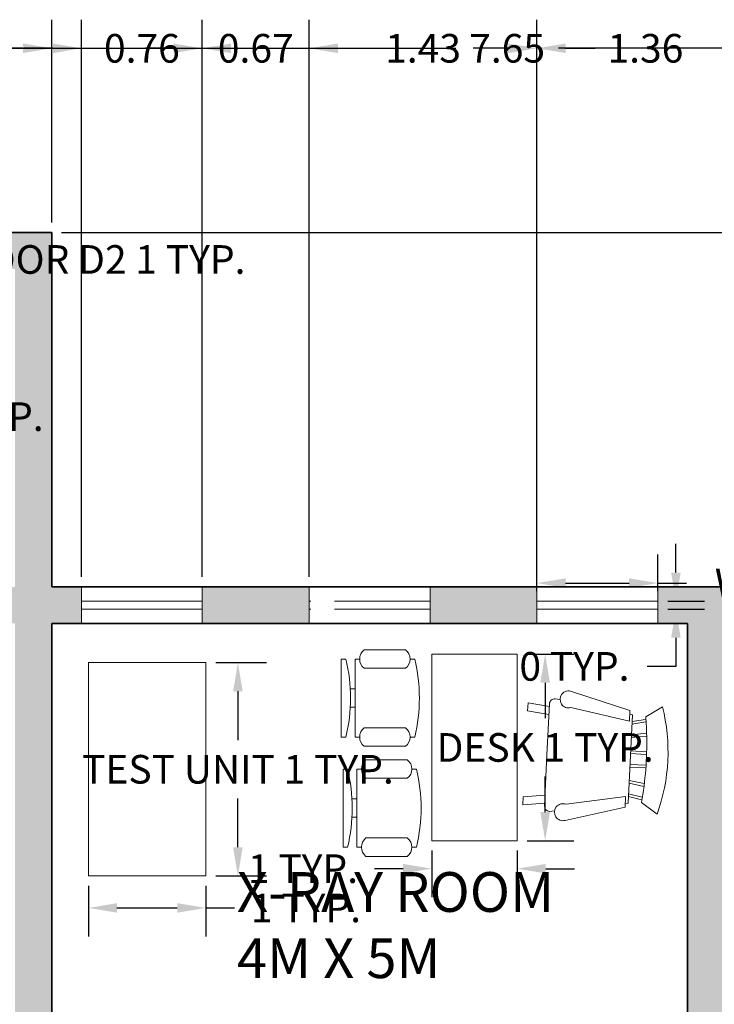
# Model space of a CAD drawing. Units: metres. Extents: x 4298.5 to 4325.2, y 2075 to 2095.8.
# Tile 33 of 35: x 4309.9 to 4314.3, y 2089.6 to 2095.8. Entities that reach past the tile are written whole.
import ezdxf

# ---------------------------------------------------------------- set-up
doc = ezdxf.new("R2010")
doc.units = ezdxf.units.M
doc.linetypes.add('ACAD_ISO02W100', pattern=[15, 12, -3])
for name, color, linetype, lineweight in [('A-ANNO-DIMS', 2, 'Continuous', 18), ('A-AREA-IDEN', 7, 'Continuous', 18), ('A-EQPM', 9, 'Continuous', 18), ('A-FURN', 15, 'Continuous', 18), ('A-GLAZ', 4, 'Continuous', 18), ('A-GLAZ-OVHD', 4, 'ACAD_ISO02W100', 13), ('A-WALL', 7, 'Continuous', 35), ('A-WALL-PATT', 252, 'Continuous', 13)]:
    doc.layers.add(name, color=color, linetype=linetype, lineweight=lineweight)
doc.styles.get("Standard").update_dxf_attribs({"font": 'arial.ttf'})
doc.dimstyles.get("Standard").update_dxf_attribs({"dimtxt": 0.18, "dimasz": 0.18, "dimexe": 0.18, "dimexo": 0.0625, "dimgap": 0.09, "dimtad": 0, "dimtih": 1, "dimtoh": 1, "dimdec": 4, "dimzin": 0, "dimdsep": 46, "dimtxsty": 'Standard', "dimcen": 0.09, "dimadec": 0, "dimazin": 0, "dimtfac": 1, "dimtdec": 4, "dimtofl": 0, "dimtmove": 0, "dimatfit": 3, "dimfxl": 1, "dimtolj": 1, "dimtzin": 0, "dimarcsym": 0})

# ---------------------------------------------------------------- blocks, each defined once
blk = doc.blocks.new('Chair - Desk')
for p, q in [((-8.5, 0), (-8.5, -1)), ((-8.5, 0), (8.5, 0)), ((8.5, 0), (8.5, -1)), ((-2, -3), (-2, -1.9355)), ((2, -1.9576), (2, -3)), ((-8.5, -3), (-8.5, -4)), ((-8.5, -3), (8.5, -3)), ((8.5, -3), (8.5, -4)), ((-10.5, -5), (-10.5, -14)), ((-6.5, -14), (-6.5, -5)), ((6.5, -5), (6.5, -14)), ((10.5, -14), (10.5, -5)), ((-8.5, -15), (-8.5, -16)), ((8.5, -15), (8.5, -16))]:
    blk.add_line(p, q)
for centre, radius, start, end in [((0, 34.625), 36.625, 256.5803, 283.4197), ((-8.5, -6.5), 2.5, 36.8699, 143.1301), ((8.5, -6.5), 2.5, 36.8699, 143.1301), ((-8.5, -12.5), 2.5, 216.8699, 323.1301), ((8.5, -12.5), 2.5, 216.8699, 323.1301), ((0, 19.625), 36.625, 256.5803, 283.4197)]:
    blk.add_arc(centre, radius, start, end)
blk = doc.blocks.new('Chair - Rocking')
for p, q in [((-8, -4.5), (-10, -1.5)), ((8, -4.5), (10, -1.5)), ((-7.5, -4.5), (-7, -7)), ((-6.5, -7), (-7.02225, -4.43)), ((-4.5, -7), (-4.96674, -4.19951)), ((-4, -7), (-4.40532, -4.16272)), ((-1.5, -4.05012), (-1.5, -7)), ((-1, -7), (-1, -4.05012)), ((1, -7), (1, -4.04655)), ((1.5, -4.05012), (1.5, -7)), ((4, -7), (4.40187, -4.18694)), ((4.5, -7), (4.96761, -4.19437)), ((6.5, -7), (7, -4.4057)), ((7.5, -4.5), (7, -7)), ((-8.23428, -6.99939), (-8.3093, -7.47958)), ((-8.23041, -7), (8.23915, -7)), ((8.31071, -7.48854), (8.23449, -7.00073)), ((-9, -7.5), (-12, -18.49999)), ((-7, -7.5), (-9, -7.5)), ((-9, -18.49999), (-7, -7.5)), ((7, -7.5), (9, -7.5)), ((9, -18.49999), (7, -7.5)), ((9, -7.5), (12, -18.49999)), ((-10.36644, -20.64523), (-10.5, -21.49999)), ((10.5, -21.49999), (10.3575, -20.58798)), ((-9, -22.49999), (-9.5, -26.49999)), ((0, -22.49999), (-9.5, -22.49999)), ((-8, -26.49999), (-7.5, -22.49999)), ((0, -22.49999), (9.5, -22.49999)), ((8, -26.49999), (7.5, -22.49999)), ((9, -22.49999), (9.5, -26.49999)), ((-9.5, -26.49999), (-8, -26.49999)), ((9.5, -26.49999), (8, -26.49999))]:
    blk.add_line(p, q)
for centre, radius, start, end in [((0, -34.08333), 34.08333, 72.93847, 107.0615), ((0, -68.25004), 64.25, 93.92211, 97.15267), ((0, -68.25004), 64.25, 82.84733, 93.92211), ((-10.5, -18.99999), 1.58114, 161.5651, 18.43495), ((10.5, -18.99999), 1.58114, 161.5651, 18.43495), ((-9.5, -21.49999), 1, 180, 270), ((9.5, -21.49999), 1, 270, 0)]:
    blk.add_arc(centre, radius, start, end)
blk = doc.blocks.new('WIN-760-GLASS-HIGH')
at = {"ltscale": 0.05}
for p, q in [((0, 0.76), (0, 0)), ((0.05, 0.76), (0.05, 0))]:
    blk.add_line(p, q, dxfattribs=at)
blk = doc.blocks.new('WIN-760-GLASS')
for p, q in [((0, 0.76), (0, 0)), ((0.05, 0.76), (0.05, 0))]:
    blk.add_line(p, q)
blk = doc.blocks.new('DESK-1175')
blk.add_lwpolyline([(0, 1.1735), (0.5376, 1.1735), (0.5376, 0), (0, 0)], close=True)
blk = doc.blocks.new('EQUIPMENT-1340')
blk.add_lwpolyline([(0, 1.3418), (0.7396, 1.3418), (0.7396, 0), (0, 0)], close=True)
blk = doc.blocks.new('*D27')
at = {"layer": 'A-ANNO-DIMS', "color": 0, "lineweight": -2, "transparency": 16777216}
for p, q in [((4313.1733, 2092.2206), (4313.1733, 2092.4521)), ((4313.9333, 2092.2206), (4313.9333, 2092.4521)), ((4313.3533, 2092.2721), (4313.7533, 2092.2721)), ((4313.9333, 2092.2721), (4314.1133, 2092.2721))]:
    blk.add_line(p, q, dxfattribs=at)
at = {"layer": 'A-ANNO-DIMS', "color": 0, "transparency": 16777216}
for points in [[(4313.3533, 2092.3021), (4313.3533, 2092.2421), (4313.1733, 2092.2721)], [(4313.7533, 2092.3021), (4313.7533, 2092.2421), (4313.9333, 2092.2721)]]:
    blk.add_solid(points, dxfattribs=at)
at = {"layer": 'Defpoints', "color": 0, "transparency": 16777216}
for p in [(4313.9333, 2092.2721), (4313.1733, 2092.1581), (4313.9333, 2092.1581)]:
    blk.add_point(p, dxfattribs=at)
at = {"layer": 'A-ANNO-DIMS', "color": 0, "transparency": 16777216, "insert": (4315.3853, 2092.2721), "char_height": 0.18, "attachment_point": 5}
blk.add_mtext('\\A1;WINDOW W3 1 TYP.', dxfattribs=at)
blk = doc.blocks.new('*D28')
at = {"layer": 'A-ANNO-DIMS', "color": 0, "lineweight": -2, "transparency": 16777216}
for p, q in [((4314.0473, 2092.3381), (4314.0473, 2092.5181)), ((4313.9958, 2092.1581), (4314.2273, 2092.1581)), ((4313.9958, 2092.1081), (4314.2273, 2092.1081)), ((4314.0473, 2091.9281), (4314.0473, 2091.7481)), ((4314.0473, 2091.7481), (4313.8673, 2091.7481))]:
    blk.add_line(p, q, dxfattribs=at)
at = {"layer": 'A-ANNO-DIMS', "color": 0, "transparency": 16777216}
for points in [[(4314.0173, 2092.3381), (4314.0773, 2092.3381), (4314.0473, 2092.1581)], [(4314.0173, 2091.9281), (4314.0773, 2091.9281), (4314.0473, 2092.1081)]]:
    blk.add_solid(points, dxfattribs=at)
at = {"layer": 'Defpoints', "color": 0, "transparency": 16777216}
for p in [(4313.9333, 2092.1581), (4313.9333, 2092.1081), (4314.0473, 2092.1081)]:
    blk.add_point(p, dxfattribs=at)
at = {"layer": 'A-ANNO-DIMS', "color": 0, "transparency": 16777216, "insert": (4313.4091, 2091.7481), "char_height": 0.18, "attachment_point": 5}
blk.add_mtext('\\A1;0 TYP.', dxfattribs=at)
blk = doc.blocks.new('*D33')
at = {"layer": 'A-ANNO-DIMS', "color": 0, "lineweight": -2, "transparency": 16777216}
for p, q in [((4309.1995, 2094.1281), (4309.1995, 2094.3081)), ((4309.1995, 2094.3081), (4309.3795, 2094.3081)), ((4309.1565, 2094.1281), (4309.3795, 2094.1281)), ((4309.1995, 2093.6047), (4309.1995, 2093.9481)), ((4309.1565, 2093.4247), (4309.3795, 2093.4247))]:
    blk.add_line(p, q, dxfattribs=at)
at = {"layer": 'A-ANNO-DIMS', "color": 0, "transparency": 16777216}
for points in [[(4309.1695, 2093.9481), (4309.2295, 2093.9481), (4309.1995, 2094.1281)], [(4309.1695, 2093.6047), (4309.2295, 2093.6047), (4309.1995, 2093.4247)]]:
    blk.add_solid(points, dxfattribs=at)
at = {"layer": 'Defpoints', "color": 0, "transparency": 16777216}
for p in [(4309.094, 2094.1281), (4309.1995, 2094.1281), (4309.094, 2093.4247)]:
    blk.add_point(p, dxfattribs=at)
at = {"layer": 'A-ANNO-DIMS', "color": 0, "transparency": 16777216, "insert": (4310.4409, 2094.3081), "char_height": 0.18, "attachment_point": 5}
blk.add_mtext('\\A1;DOOR D2 1 TYP.', dxfattribs=at)
blk = doc.blocks.new('*D34')
at = {"layer": 'A-ANNO-DIMS', "color": 0, "lineweight": -2, "transparency": 16777216}
for p, q in [((4308.3906, 2093.3622), (4308.3906, 2093.1392)), ((4309.094, 2093.3622), (4309.094, 2093.1392)), ((4308.5706, 2093.3192), (4308.914, 2093.3192)), ((4309.094, 2093.3192), (4309.274, 2093.3192))]:
    blk.add_line(p, q, dxfattribs=at)
at = {"layer": 'A-ANNO-DIMS', "color": 0, "transparency": 16777216}
for points in [[(4308.5706, 2093.3492), (4308.5706, 2093.2892), (4308.3906, 2093.3192)], [(4308.914, 2093.3492), (4308.914, 2093.2892), (4309.094, 2093.3192)]]:
    blk.add_solid(points, dxfattribs=at)
at = {"layer": 'Defpoints', "color": 0, "transparency": 16777216}
for p in [(4308.3906, 2093.4247), (4309.094, 2093.4247), (4309.094, 2093.3192)]:
    blk.add_point(p, dxfattribs=at)
at = {"layer": 'A-ANNO-DIMS', "color": 0, "transparency": 16777216, "insert": (4309.7237, 2093.3192), "char_height": 0.18, "attachment_point": 5}
blk.add_mtext('\\A1;1 TYP.', dxfattribs=at)
blk = doc.blocks.new('*D37')
at = {"layer": 'A-ANNO-DIMS', "color": 0, "lineweight": -2, "transparency": 16777216}
for p, q in [((4313.1112, 2091.825), (4313.4047, 2091.825)), ((4313.2247, 2091.645), (4313.2247, 2091.4213)), ((4313.2247, 2090.8315), (4313.2247, 2091.0551)), ((4313.1112, 2090.6515), (4313.4047, 2090.6515))]:
    blk.add_line(p, q, dxfattribs=at)
at = {"layer": 'A-ANNO-DIMS', "color": 0, "transparency": 16777216}
for points in [[(4313.1947, 2091.645), (4313.2547, 2091.645), (4313.2247, 2091.825)], [(4313.1947, 2090.8315), (4313.2547, 2090.8315), (4313.2247, 2090.6515)]]:
    blk.add_solid(points, dxfattribs=at)
at = {"layer": 'Defpoints', "color": 0, "transparency": 16777216}
for p in [(4313.0487, 2091.825), (4313.0487, 2090.6515), (4313.2247, 2090.6515)]:
    blk.add_point(p, dxfattribs=at)
at = {"layer": 'A-ANNO-DIMS', "color": 0, "transparency": 16777216, "insert": (4313.2247, 2091.2382), "char_height": 0.18, "attachment_point": 5}
blk.add_mtext('\\A1;DESK 1 TYP.', dxfattribs=at)
blk = doc.blocks.new('*D38')
at = {"layer": 'A-ANNO-DIMS', "color": 0, "lineweight": -2, "transparency": 16777216}
for p, q in [((4312.5111, 2090.589), (4312.5111, 2090.2955)), ((4313.0487, 2090.589), (4313.0487, 2090.2955)), ((4312.3311, 2090.4755), (4312.1511, 2090.4755)), ((4313.2287, 2090.4755), (4313.4087, 2090.4755))]:
    blk.add_line(p, q, dxfattribs=at)
at = {"layer": 'A-ANNO-DIMS', "color": 0, "transparency": 16777216}
for points in [[(4312.3311, 2090.5055), (4312.3311, 2090.4455), (4312.5111, 2090.4755)], [(4313.2287, 2090.5055), (4313.2287, 2090.4455), (4313.0487, 2090.4755)]]:
    blk.add_solid(points, dxfattribs=at)
at = {"layer": 'Defpoints', "color": 0, "transparency": 16777216}
for p in [(4312.5111, 2090.6515), (4313.0487, 2090.6515), (4312.5111, 2090.4755)]:
    blk.add_point(p, dxfattribs=at)
at = {"layer": 'A-ANNO-DIMS', "color": 0, "transparency": 16777216, "insert": (4311.7014, 2090.4755), "char_height": 0.18, "attachment_point": 5}
blk.add_mtext('\\A1;1 TYP.', dxfattribs=at)
blk = doc.blocks.new('*D43')
at = {"layer": 'A-ANNO-DIMS', "color": 0, "lineweight": -2, "transparency": 16777216}
for p, q in [((4311.1532, 2091.7717), (4311.4719, 2091.7717)), ((4311.2919, 2091.5917), (4311.2919, 2091.2839)), ((4311.2919, 2090.6099), (4311.2919, 2090.9177)), ((4311.1532, 2090.4299), (4311.4719, 2090.4299))]:
    blk.add_line(p, q, dxfattribs=at)
at = {"layer": 'A-ANNO-DIMS', "color": 0, "transparency": 16777216}
for points in [[(4311.2619, 2091.5917), (4311.3219, 2091.5917), (4311.2919, 2091.7717)], [(4311.2619, 2090.6099), (4311.3219, 2090.6099), (4311.2919, 2090.4299)]]:
    blk.add_solid(points, dxfattribs=at)
at = {"layer": 'Defpoints', "color": 0, "transparency": 16777216}
for p in [(4311.0907, 2091.7717), (4311.2919, 2091.7717), (4311.0907, 2090.4299)]:
    blk.add_point(p, dxfattribs=at)
at = {"layer": 'A-ANNO-DIMS', "color": 0, "transparency": 16777216, "insert": (4311.2919, 2091.1008), "char_height": 0.18, "attachment_point": 5}
blk.add_mtext('\\A1;TEST UNIT 1 TYP.', dxfattribs=at)
blk = doc.blocks.new('*D44')
at = {"layer": 'A-ANNO-DIMS', "color": 0, "lineweight": -2, "transparency": 16777216}
for p, q in [((4310.3511, 2090.3674), (4310.3511, 2090.0486)), ((4311.0907, 2090.3674), (4311.0907, 2090.0486)), ((4310.5311, 2090.2286), (4310.9107, 2090.2286)), ((4311.0907, 2090.2286), (4311.2707, 2090.2286))]:
    blk.add_line(p, q, dxfattribs=at)
at = {"layer": 'A-ANNO-DIMS', "color": 0, "transparency": 16777216}
for points in [[(4310.5311, 2090.2586), (4310.5311, 2090.1986), (4310.3511, 2090.2286)], [(4310.9107, 2090.2586), (4310.9107, 2090.1986), (4311.0907, 2090.2286)]]:
    blk.add_solid(points, dxfattribs=at)
at = {"layer": 'Defpoints', "color": 0, "transparency": 16777216}
for p in [(4310.3511, 2090.4299), (4311.0907, 2090.4299), (4311.0907, 2090.2286)]:
    blk.add_point(p, dxfattribs=at)
at = {"layer": 'A-ANNO-DIMS', "color": 0, "transparency": 16777216, "insert": (4311.7204, 2090.2286), "char_height": 0.18, "attachment_point": 5}
blk.add_mtext('\\A1;1 TYP.', dxfattribs=at)
blk = doc.blocks.new('*D48')
at = {"layer": 'A-ANNO-DIMS', "color": 0, "lineweight": -2, "transparency": 16777216}
for p, q in [((4310.1831, 2094.4781), (4324.7671, 2094.4781)), ((4324.5871, 2094.2981), (4324.5871, 2085.585)), ((4324.5871, 2076.5081), (4324.5871, 2085.2212)), ((4316.8731, 2076.3281), (4324.7671, 2076.3281))]:
    blk.add_line(p, q, dxfattribs=at)
at = {"layer": 'A-ANNO-DIMS', "color": 0, "transparency": 16777216}
for points in [[(4324.5571, 2094.2981), (4324.6171, 2094.2981), (4324.5871, 2094.4781)], [(4324.5571, 2076.5081), (4324.6171, 2076.5081), (4324.5871, 2076.3281)]]:
    blk.add_solid(points, dxfattribs=at)
at = {"layer": 'Defpoints', "color": 0, "transparency": 16777216}
for p in [(4310.1206, 2094.4781), (4316.8106, 2076.3281), (4324.5871, 2076.3281)]:
    blk.add_point(p, dxfattribs=at)
at = {"layer": 'A-ANNO-DIMS', "color": 0, "transparency": 16777216, "insert": (4324.5871, 2085.4031), "char_height": 0.18, "attachment_point": 5}
blk.add_mtext('\\A1;18.15', dxfattribs=at)
blk = doc.blocks.new('*D50')
at = {"layer": 'A-ANNO-DIMS', "color": 0, "lineweight": -2, "transparency": 16777216}
for p, q in [((4305.6606, 2094.5406), (4305.6606, 2095.8166)), ((4310.1206, 2094.5406), (4310.1206, 2095.8166)), ((4305.8406, 2095.6366), (4307.5632, 2095.6366)), ((4309.9406, 2095.6366), (4308.2179, 2095.6366))]:
    blk.add_line(p, q, dxfattribs=at)
at = {"layer": 'A-ANNO-DIMS', "color": 0, "transparency": 16777216}
for points in [[(4305.8406, 2095.6666), (4305.8406, 2095.6066), (4305.6606, 2095.6366)], [(4309.9406, 2095.6666), (4309.9406, 2095.6066), (4310.1206, 2095.6366)]]:
    blk.add_solid(points, dxfattribs=at)
at = {"layer": 'Defpoints', "color": 0, "transparency": 16777216}
for p in [(4310.1206, 2095.6366), (4305.6606, 2094.4781), (4310.1206, 2094.4781)]:
    blk.add_point(p, dxfattribs=at)
at = {"layer": 'A-ANNO-DIMS', "color": 0, "transparency": 16777216, "insert": (4307.8906, 2095.6366), "char_height": 0.18, "attachment_point": 5}
blk.add_mtext('\\A1;4.46', dxfattribs=at)
blk = doc.blocks.new('*D53')
at = {"layer": 'A-ANNO-DIMS', "color": 0, "lineweight": -2, "transparency": 16777216}
for p, q in [((4309.1606, 2076.3906), (4309.1606, 2095.8166)), ((4316.8106, 2076.3906), (4316.8106, 2095.8166)), ((4309.3406, 2095.6366), (4312.6619, 2095.6366)), ((4316.6306, 2095.6366), (4313.3093, 2095.6366))]:
    blk.add_line(p, q, dxfattribs=at)
at = {"layer": 'A-ANNO-DIMS', "color": 0, "transparency": 16777216}
for points in [[(4309.3406, 2095.6666), (4309.3406, 2095.6066), (4309.1606, 2095.6366)], [(4316.6306, 2095.6666), (4316.6306, 2095.6066), (4316.8106, 2095.6366)]]:
    blk.add_solid(points, dxfattribs=at)
at = {"layer": 'Defpoints', "color": 0, "transparency": 16777216}
for p in [(4316.8106, 2095.6366), (4309.1606, 2076.3281), (4316.8106, 2076.3281)]:
    blk.add_point(p, dxfattribs=at)
at = {"layer": 'A-ANNO-DIMS', "color": 0, "transparency": 16777216, "insert": (4312.9856, 2095.6366), "char_height": 0.18, "attachment_point": 5}
blk.add_mtext('\\A1;7.65', dxfattribs=at)
blk = doc.blocks.new('*D65')
at = {"layer": 'A-ANNO-DIMS', "color": 0, "lineweight": -2, "transparency": 16777216}
for p, q in [((4310.307848, 2092.310556), (4310.307848, 2095.816556)), ((4311.067848, 2092.310556), (4311.067848, 2095.816556)), ((4310.127848, 2095.636556), (4309.947848, 2095.636556)), ((4311.247848, 2095.636556), (4311.427848, 2095.636556))]:
    blk.add_line(p, q, dxfattribs=at)
at = {"layer": 'A-ANNO-DIMS', "color": 0, "transparency": 16777216}
for points in [[(4310.127848, 2095.666556), (4310.127848, 2095.606556), (4310.307848, 2095.636556)], [(4311.247848, 2095.666556), (4311.247848, 2095.606556), (4311.067848, 2095.636556)]]:
    blk.add_solid(points, dxfattribs=at)
at = {"layer": 'Defpoints', "color": 0, "transparency": 16777216}
for p in [(4311.067848, 2095.636556), (4310.307848, 2092.248056), (4311.067848, 2092.248056)]:
    blk.add_point(p, dxfattribs=at)
at = {"layer": 'A-ANNO-DIMS', "color": 0, "transparency": 16777216, "insert": (4310.687848, 2095.636556), "char_height": 0.18, "attachment_point": 5}
blk.add_mtext('\\A1;0.76', dxfattribs=at)
blk = doc.blocks.new('*D66')
at = {"layer": 'A-ANNO-DIMS', "color": 0, "lineweight": -2, "transparency": 16777216}
for p, q in [((4311.0678, 2092.3106), (4311.0678, 2095.8166)), ((4311.7406, 2092.3106), (4311.7406, 2095.8166)), ((4310.8878, 2095.6366), (4310.7078, 2095.6366)), ((4311.9206, 2095.6366), (4312.1006, 2095.6366))]:
    blk.add_line(p, q, dxfattribs=at)
at = {"layer": 'A-ANNO-DIMS', "color": 0, "transparency": 16777216}
for points in [[(4310.8878, 2095.6666), (4310.8878, 2095.6066), (4311.0678, 2095.6366)], [(4311.9206, 2095.6666), (4311.9206, 2095.6066), (4311.7406, 2095.6366)]]:
    blk.add_solid(points, dxfattribs=at)
at = {"layer": 'Defpoints', "color": 0, "transparency": 16777216}
for p in [(4311.7406, 2095.6366), (4311.0678, 2092.2481), (4311.7406, 2092.2481)]:
    blk.add_point(p, dxfattribs=at)
at = {"layer": 'A-ANNO-DIMS', "color": 0, "transparency": 16777216, "insert": (4311.4042, 2095.6366), "char_height": 0.18, "attachment_point": 5}
blk.add_mtext('\\A1;0.67', dxfattribs=at)
blk = doc.blocks.new('*D67')
at = {"layer": 'A-ANNO-DIMS', "color": 0, "lineweight": -2, "transparency": 16777216}
for p, q in [((4311.7406, 2092.3106), (4311.7406, 2095.8166)), ((4313.1733, 2092.3106), (4313.1733, 2095.8166)), ((4311.9206, 2095.6366), (4312.1416, 2095.6366)), ((4312.9933, 2095.6366), (4312.7722, 2095.6366))]:
    blk.add_line(p, q, dxfattribs=at)
at = {"layer": 'A-ANNO-DIMS', "color": 0, "transparency": 16777216}
for points in [[(4311.9206, 2095.6666), (4311.9206, 2095.6066), (4311.7406, 2095.6366)], [(4312.9933, 2095.6666), (4312.9933, 2095.6066), (4313.1733, 2095.6366)]]:
    blk.add_solid(points, dxfattribs=at)
at = {"layer": 'Defpoints', "color": 0, "transparency": 16777216}
for p in [(4313.1733, 2095.6366), (4311.7406, 2092.2481), (4313.1733, 2092.2481)]:
    blk.add_point(p, dxfattribs=at)
at = {"layer": 'A-ANNO-DIMS', "color": 0, "transparency": 16777216, "insert": (4312.4569, 2095.6366), "char_height": 0.18, "attachment_point": 5}
blk.add_mtext('\\A1;1.43', dxfattribs=at)
blk = doc.blocks.new('*D68')
at = {"layer": 'A-ANNO-DIMS', "color": 0, "lineweight": -2, "transparency": 16777216}
for p, q in [((4313.1733, 2092.3106), (4313.1733, 2095.8166)), ((4314.5378, 2092.3106), (4314.5378, 2095.8166)), ((4313.3533, 2095.6366), (4313.5403, 2095.6366)), ((4314.3578, 2095.6366), (4314.1708, 2095.6366))]:
    blk.add_line(p, q, dxfattribs=at)
at = {"layer": 'A-ANNO-DIMS', "color": 0, "transparency": 16777216}
for points in [[(4313.3533, 2095.6666), (4313.3533, 2095.6066), (4313.1733, 2095.6366)], [(4314.3578, 2095.6666), (4314.3578, 2095.6066), (4314.5378, 2095.6366)]]:
    blk.add_solid(points, dxfattribs=at)
at = {"layer": 'Defpoints', "color": 0, "transparency": 16777216}
for p in [(4314.5378, 2095.6366), (4313.1733, 2092.2481), (4314.5378, 2092.2481)]:
    blk.add_point(p, dxfattribs=at)
at = {"layer": 'A-ANNO-DIMS', "color": 0, "transparency": 16777216, "insert": (4313.8556, 2095.6366), "char_height": 0.18, "attachment_point": 5}
blk.add_mtext('\\A1;1.36', dxfattribs=at)

msp = doc.modelspace()

# ---------------------------------------------------------------- hatches: boundary and pattern name
at = {"layer": 'A-WALL-PATT'}
h = msp.add_hatch(color=256, dxfattribs=at)
h.dxf.hatch_style = 1
h.paths.add_polyline_path([(4308.7606, 2094.4781), (4308.1606, 2094.4781), (4307.4606, 2094.4781), (4307.4606, 2094.2481), (4308.2706, 2094.2481), (4308.2706, 2094.1281), (4308.3906, 2094.1281), (4308.3906, 2094.2481), (4308.7606, 2094.2481)])
h.paths.add_polyline_path([(4310.1206, 2094.4781), (4309.5206, 2094.4781), (4309.5206, 2094.2481), (4309.8906, 2094.2481), (4309.8906, 2092.2481), (4308.3906, 2092.2481), (4308.3906, 2093.4281), (4308.2706, 2093.4281), (4308.2706, 2092.0181), (4309.8906, 2092.0181), (4309.8906, 2087.0181), (4309.7706, 2087.0181), (4309.7706, 2086.7881), (4309.8906, 2086.7881), (4311.9406, 2086.7881), (4311.9406, 2087.0181), (4310.1206, 2087.0181), (4310.1206, 2089.0181), (4310.2406, 2089.0181), (4310.2406, 2089.1381), (4310.1206, 2089.1381), (4310.1206, 2092.0181), (4310.3078, 2092.0181), (4310.3078, 2092.2481), (4310.1206, 2092.2481)])
h.paths.add_polyline_path([(4311.7406, 2092.2481), (4311.0678, 2092.2481), (4311.0678, 2092.0181), (4311.7406, 2092.0181)], flags=17)
h.paths.add_polyline_path([(4313.1733, 2092.2481), (4312.5006, 2092.2481), (4312.5006, 2092.0181), (4313.1733, 2092.0181)])
h.paths.add_polyline_path([(4314.5378, 2092.2481), (4314.1206, 2092.2481), (4313.9333, 2092.2481), (4313.9333, 2092.0181), (4314.1206, 2092.0181), (4314.1206, 2087.0181), (4314.0006, 2087.0181), (4314.0006, 2086.7881), (4314.1206, 2086.7881), (4315.5718, 2086.7881), (4315.5718, 2087.0181), (4314.3506, 2087.0181), (4314.3506, 2092.0181), (4314.5378, 2092.0181)])
h.paths.add_polyline_path([(4315.9706, 2092.2481), (4315.2978, 2092.2481), (4315.2978, 2092.0181), (4315.9706, 2092.0181)])
h.paths.add_polyline_path([(4317.4033, 2092.2481), (4316.7306, 2092.2481), (4316.7306, 2092.0181), (4317.4033, 2092.0181)])
h.paths.add_polyline_path([(4318.9506, 2092.2481), (4318.3506, 2092.2481), (4318.1633, 2092.2481), (4318.1633, 2092.0181), (4318.3506, 2092.0181), (4318.3506, 2091.8981), (4318.5806, 2091.8981), (4318.5806, 2092.0181), (4318.9506, 2092.0181)])
h.paths.add_polyline_path([(4321.0106, 2092.2481), (4319.7106, 2092.2481), (4319.7106, 2092.0181), (4320.0806, 2092.0181), (4320.0806, 2090.0181), (4318.5806, 2090.0181), (4318.5806, 2091.1981), (4318.3506, 2091.1981), (4318.3506, 2090.0181), (4318.3506, 2087.0181), (4318.2306, 2087.0181), (4318.2306, 2086.7881), (4318.3506, 2086.7881), (4318.3506, 2086.3081), (4318.5806, 2086.3081), (4318.5806, 2089.7881), (4321.7806, 2089.7881), (4321.7806, 2090.0181), (4320.2006, 2090.0181), (4320.2006, 2092.0181), (4321.0106, 2092.0181)])
h.paths.add_polyline_path([(4322.8106, 2092.2481), (4321.7706, 2092.2481), (4321.7706, 2092.0181), (4322.5806, 2092.0181), (4322.5806, 2091.2831), (4322.8106, 2091.2831)])
h.paths.add_polyline_path([(4322.8106, 2090.5231), (4322.5806, 2090.5231), (4322.5806, 2089.7881), (4322.5806, 2089.5254), (4322.8106, 2089.5254), (4322.8106, 2090.0181)])
h.paths.add_polyline_path([(4322.8106, 2088.7654), (4322.5806, 2088.7654), (4322.5806, 2087.6681), (4322.8106, 2087.6681)])
h.paths.add_polyline_path([(4322.8106, 2086.9081), (4322.5806, 2086.9081), (4322.5806, 2085.8107), (4322.8106, 2085.8107)])
h.paths.add_polyline_path([(4322.8106, 2085.0507), (4322.5806, 2085.0507), (4322.5806, 2084.7881), (4318.5806, 2084.7881), (4318.5806, 2085.0581), (4318.5806, 2085.4081), (4318.3506, 2085.4081), (4318.3506, 2084.5581), (4318.3506, 2080.8581), (4318.4706, 2080.8581), (4318.4706, 2082.3281), (4319.2606, 2082.3281), (4319.2606, 2082.5581), (4318.5806, 2082.5581), (4318.5806, 2084.5581), (4320.0806, 2084.5581), (4320.0806, 2083.9381), (4320.3106, 2083.9381), (4320.3106, 2084.5581), (4322.8106, 2084.5581)])
h.paths.add_polyline_path([(4320.3106, 2083.1781), (4320.0806, 2083.1781), (4320.0806, 2082.5581), (4319.9606, 2082.5581), (4319.9606, 2082.3281), (4320.0806, 2082.3281), (4320.0806, 2081.5731), (4320.3106, 2081.5731)], flags=17)
h.paths.add_polyline_path([(4320.3106, 2080.8131), (4320.0806, 2080.8131), (4320.0806, 2080.0581), (4318.4286, 2080.0581), (4318.4286, 2079.8281), (4320.3106, 2079.8281)])
h.paths.add_polyline_path([(4317.3506, 2085.2881), (4316.5718, 2085.2881), (4316.5718, 2085.0581), (4317.3506, 2085.0581)])
h.paths.add_polyline_path([(4315.5718, 2085.2881), (4314.8434, 2085.2881), (4314.8434, 2085.0581), (4315.5718, 2085.0581)])
h.paths.add_polyline_path([(4313.8434, 2085.2881), (4312.9406, 2085.2881), (4312.9406, 2085.0581), (4313.8434, 2085.0581)])
h.paths.add_polyline_path([(4311.9406, 2085.2881), (4311.4406, 2085.2881), (4311.4406, 2085.0581), (4311.9406, 2085.0581)])
h.paths.add_polyline_path([(4317.3306, 2087.0181), (4316.5718, 2087.0181), (4316.5718, 2086.7881), (4317.3306, 2086.7881)])
h.paths.add_polyline_path([(4313.1006, 2089.1381), (4311.1406, 2089.1381), (4311.1406, 2089.0181), (4312.9806, 2089.0181), (4312.9806, 2087.0181), (4312.9406, 2087.0181), (4312.9406, 2086.7881), (4313.1006, 2086.7881), (4313.1006, 2087.0181)])
h.paths.add_polyline_path([(4307.5515, 2087.0181), (4305.8906, 2087.0181), (4305.8906, 2092.2481), (4305.8906, 2094.2481), (4306.7006, 2094.2481), (4306.7006, 2094.4781), (4305.6606, 2094.4781), (4305.6606, 2092.2481), (4305.2906, 2092.2481), (4305.2906, 2092.0181), (4305.6606, 2092.0181), (4305.6606, 2090.0181), (4304.1606, 2090.0181), (4304.1606, 2091.1981), (4304.0406, 2091.1981), (4304.0406, 2089.9081), (4301.5606, 2089.9081), (4301.5606, 2089.7881), (4304.0406, 2089.7881), (4305.6606, 2089.7881), (4305.6606, 2086.6381), (4305.8906, 2086.6381), (4305.8906, 2086.7881), (4307.5515, 2086.7881)])
h.paths.add_polyline_path([(4307.5515, 2085.2881), (4305.8906, 2085.2881), (4305.8906, 2085.4381), (4305.6606, 2085.4381), (4305.6606, 2084.7881), (4305.2906, 2084.7881), (4305.2906, 2084.5581), (4305.6606, 2084.5581), (4305.6606, 2084.02), (4305.8906, 2084.02), (4305.8906, 2084.5581), (4305.8906, 2085.0581), (4307.5515, 2085.0581)])
h.paths.add_polyline_path([(4310.2406, 2085.2881), (4308.5515, 2085.2881), (4308.5515, 2085.0581), (4310.2406, 2085.0581)])
h.paths.add_polyline_path([(4317.4286, 2080.0581), (4316.5718, 2080.0581), (4316.5718, 2079.8281), (4317.4286, 2079.8281)])
h.paths.add_polyline_path([(4315.5718, 2080.0581), (4314.8434, 2080.0581), (4314.8434, 2079.8281), (4315.5718, 2079.8281)])
h.paths.add_polyline_path([(4313.8434, 2080.0581), (4312.9406, 2080.0581), (4312.9406, 2079.8281), (4313.8434, 2079.8281)])
h.paths.add_polyline_path([(4311.9406, 2080.0581), (4311.4406, 2080.0581), (4311.4406, 2079.8281), (4311.9406, 2079.8281)])
h.paths.add_polyline_path([(4310.2406, 2080.0581), (4310.1206, 2080.0581), (4310.1206, 2084.0381), (4309.8906, 2084.0381), (4309.8906, 2080.0581), (4309.1606, 2080.0581), (4309.1606, 2079.8281), (4310.2406, 2079.8281)])
h.paths.add_polyline_path([(4308.1606, 2080.0581), (4307.5106, 2080.0581), (4307.5106, 2080.1781), (4307.3906, 2080.1781), (4307.3906, 2080.0581), (4305.8906, 2080.0581), (4305.8906, 2080.567), (4305.6606, 2080.567), (4305.6606, 2079.8281), (4308.1606, 2079.8281)])
h.paths.add_polyline_path([(4307.5106, 2081.9381), (4309.0906, 2081.9381), (4309.0906, 2082.0581), (4305.8906, 2082.0581), (4305.8906, 2083.26), (4305.6606, 2083.26), (4305.6606, 2081.327), (4305.8906, 2081.327), (4305.8906, 2081.9381), (4307.3906, 2081.9381), (4307.3906, 2080.8781), (4307.5106, 2080.8781)])
h.paths.add_polyline_path([(4304.5306, 2084.7881), (4302.7306, 2084.7881), (4302.7306, 2084.5581), (4304.5306, 2084.5581)])
h.paths.add_polyline_path([(4301.9706, 2084.7881), (4300.6606, 2084.7881), (4300.6606, 2085.0249), (4300.4306, 2085.0249), (4300.4306, 2084.5581), (4301.9706, 2084.5581)])
h.paths.add_polyline_path([(4300.6606, 2086.8843), (4300.4306, 2086.8843), (4300.4306, 2085.7849), (4300.6606, 2085.7849)])
h.paths.add_polyline_path([(4300.6606, 2089.1618), (4300.4306, 2089.1618), (4300.4306, 2087.6443), (4300.6606, 2087.6443)])
h.paths.add_polyline_path([(4300.6606, 2091.0212), (4300.4306, 2091.0212), (4300.4306, 2089.9218), (4300.6606, 2089.9218)])
h.paths.add_polyline_path([(4300.6606, 2092.0181), (4301.9706, 2092.0181), (4301.9706, 2092.2481), (4300.4306, 2092.2481), (4300.4306, 2091.7812), (4300.6606, 2091.7812)])
h.paths.add_polyline_path([(4304.5306, 2092.2481), (4302.7306, 2092.2481), (4302.7306, 2092.0181), (4304.0406, 2092.0181), (4304.0406, 2091.8981), (4304.1606, 2091.8981), (4304.1606, 2092.0181), (4304.5306, 2092.0181)], flags=17)

# ---------------------------------------------------------------- linework, layer by layer
at = {"layer": 'A-GLAZ'}
for p, q in [((4310.3078, 2092.0181), (4310.3078, 2092.2481)), ((4311.0678, 2092.0181), (4311.0678, 2092.2481)), ((4311.7406, 2092.0181), (4311.7406, 2092.2481)), ((4312.5006, 2092.0181), (4312.5006, 2092.2481)), ((4313.1733, 2092.0181), (4313.1733, 2092.2481)), ((4313.9333, 2092.0181), (4313.9333, 2092.2481))]:
    msp.add_line(p, q, dxfattribs=at)
at = {"layer": 'A-WALL'}
for p, q in [((4310.1206, 2094.4781), (4308.1606, 2094.4781)), ((4310.1206, 2092.2481), (4310.1206, 2094.4781)), ((4314.1206, 2092.2481), (4310.1206, 2092.2481)), ((4318.3506, 2092.2481), (4314.1206, 2092.2481)), ((4314.1206, 2092.0181), (4310.1206, 2092.0181)), ((4310.1206, 2092.0181), (4310.1206, 2089.1381)), ((4314.1206, 2092.0181), (4314.1206, 2087.0181))]:
    msp.add_line(p, q, dxfattribs=at)

# ---------------------------------------------------------------- block references
at = {"layer": 'A-EQPM'}
msp.add_blockref('EQUIPMENT-1340', (4310.3511, 2090.4299), dxfattribs=at)
at = {"layer": 'A-FURN'}
for name, p, xscale, yscale, zscale, rotation in [('Chair - Desk', (4311.9424, 2091.5487), 0.0288995186862949, 0.0288995186862949, 0.0288995186862949, 89.99999999999999), ('Chair - Rocking', (4313.9965, 2091.1536), 0.0338365474760119, 0.0338365474760119, 0.0338365474760119, 267.1375936308194), ('Chair - Desk', (4311.9532, 2090.8564), 0.0288995186862949, 0.0288995186862949, 0.0288995186862949, 89.99999999999999)]:
    msp.add_blockref(name, p, dxfattribs=dict(at, xscale=xscale, yscale=yscale, zscale=zscale, rotation=rotation))
at = {"layer": 'A-FURN', "rotation": 180}
msp.add_blockref('DESK-1175', (4313.0487, 2091.825), dxfattribs=at)
at = {"layer": 'A-GLAZ'}
for p, rotation in [((4310.3078, 2092.1581), 269.9999999999452), ((4313.1733, 2092.1581), 269.9999999999362)]:
    msp.add_blockref('WIN-760-GLASS', p, dxfattribs=dict(at, rotation=rotation))
at = {"layer": 'A-GLAZ-OVHD', "rotation": 269.9999999999317}
msp.add_blockref('WIN-760-GLASS-HIGH', (4311.7406, 2092.1581), dxfattribs=at)

# ---------------------------------------------------------------- texts
at = {"layer": 'A-AREA-IDEN', "insert": (4311.2859, 2090.4538), "char_height": 0.25, "attachment_point": 1}
msp.add_mtext_dynamic_manual_height_columns('X-RAY ROOM\\P4M X 5M', width=2.22034, gutter_width=12.5, heights=[0], dxfattribs=at)

# ---------------------------------------------------------------- dimensions: what is measured, and where the dimension line sits
at = {"layer": 'A-ANNO-DIMS'}
for base, p1, p2, picture, middle in [((4310.1206, 2095.6366), (4305.6606, 2094.4781), (4310.1206, 2094.4781), '*D50', (4307.8906, 2095.6366)), ((4316.8106, 2095.6366), (4309.1606, 2076.3281), (4316.8106, 2076.3281), '*D53', (4312.9856, 2095.6366)), ((4311.0678, 2095.6366), (4310.3078, 2092.2481), (4311.0678, 2092.2481), '*D65', (4310.6878, 2095.6366)), ((4311.7406, 2095.6366), (4311.0678, 2092.2481), (4311.7406, 2092.2481), '*D66', (4311.4042, 2095.6366)), ((4313.1733, 2095.6366), (4311.7406, 2092.2481), (4313.1733, 2092.2481), '*D67', (4312.4569, 2095.6366)), ((4314.5378, 2095.6366), (4313.1733, 2092.2481), (4314.5378, 2092.2481), '*D68', (4313.8556, 2095.6366))]:
    dim = msp.add_linear_dim(base=base, p1=p1, p2=p2, dimstyle='Standard', override={"dimdec": 2, "dimlfac": 1, "dimrnd": 0, "dimzin": 0, "dimdsep": 46, "dimlunit": 2}, dxfattribs=at)
    dim.commit()
    dim.dimension.update_dxf_attribs({"geometry": picture, "text_midpoint": middle})
for base, p1, p2, angle, text, picture, middle in [((4309.1995, 2094.1281), (4309.094, 2093.4247), (4309.094, 2094.1281), 90, 'DOOR D2 <> TYP.', '*D33', (4310.4409, 2094.3081)), ((4314.0473, 2092.1081), (4313.9333, 2092.1581), (4313.9333, 2092.1081), 270, '<> TYP.', '*D28', (4313.4091, 2091.7481)), ((4313.2247, 2090.6515), (4313.0487, 2091.825), (4313.0487, 2090.6515), 270, 'DESK <> TYP.', '*D37', (4313.2247, 2091.2382)), ((4311.2919, 2091.7717), (4311.0907, 2090.4299), (4311.0907, 2091.7717), 90, 'TEST UNIT <> TYP.', '*D43', (4311.2919, 2091.1008)), ((4312.5111, 2090.4755), (4313.0487, 2090.6515), (4312.5111, 2090.6515), 180, '<> TYP.', '*D38', (4311.7014, 2090.4755))]:
    dim = msp.add_linear_dim(base=base, p1=p1, p2=p2, angle=angle, text=text, dimstyle='Standard', override={"dimdec": 0, "dimlfac": 1, "dimrnd": 0, "dimzin": 0, "dimdsep": 46, "dimlunit": 2}, dxfattribs=at)
    dim.commit()
    dim.dimension.update_dxf_attribs({"geometry": picture, "text_midpoint": middle})
dim = msp.add_linear_dim(base=(4324.5871, 2076.3281), p1=(4310.1206, 2094.4781), p2=(4316.8106, 2076.3281), angle=90, dimstyle='Standard', override={"dimdec": 2, "dimlfac": 1, "dimrnd": 0, "dimzin": 0, "dimdsep": 46, "dimlunit": 2}, dxfattribs=at)
dim.commit()
dim.dimension.update_dxf_attribs({"geometry": '*D48', "text_midpoint": (4324.5871, 2085.4031)})
for base, p1, p2, text, picture, middle in [((4309.094, 2093.3192), (4308.3906, 2093.4247), (4309.094, 2093.4247), '<> TYP.', '*D34', (4309.7237, 2093.3192)), ((4313.9333, 2092.2721), (4313.1733, 2092.1581), (4313.9333, 2092.1581), 'WINDOW W3 <> TYP.', '*D27', (4315.3853, 2092.2721)), ((4311.0907, 2090.2286), (4310.3511, 2090.4299), (4311.0907, 2090.4299), '<> TYP.', '*D44', (4311.7204, 2090.2286))]:
    dim = msp.add_linear_dim(base=base, p1=p1, p2=p2, text=text, dimstyle='Standard', override={"dimdec": 0, "dimlfac": 1, "dimrnd": 0, "dimzin": 0, "dimdsep": 46, "dimlunit": 2}, dxfattribs=at)
    dim.commit()
    dim.dimension.update_dxf_attribs({"geometry": picture, "text_midpoint": middle})

doc.saveas('drawing.dxf')
